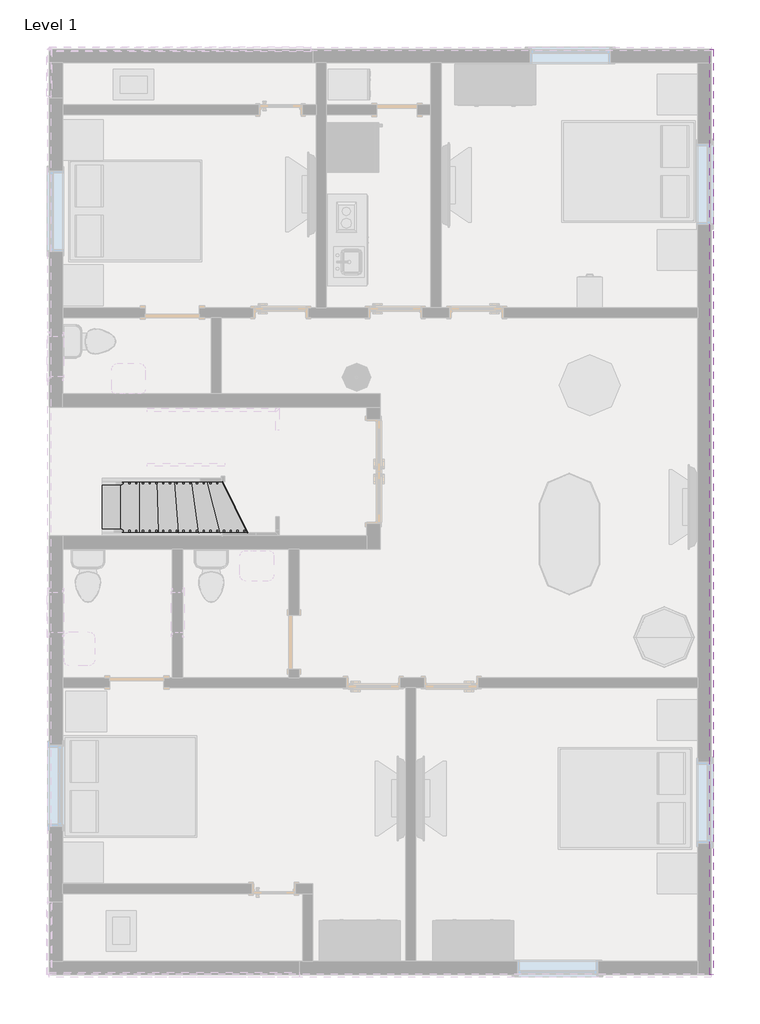
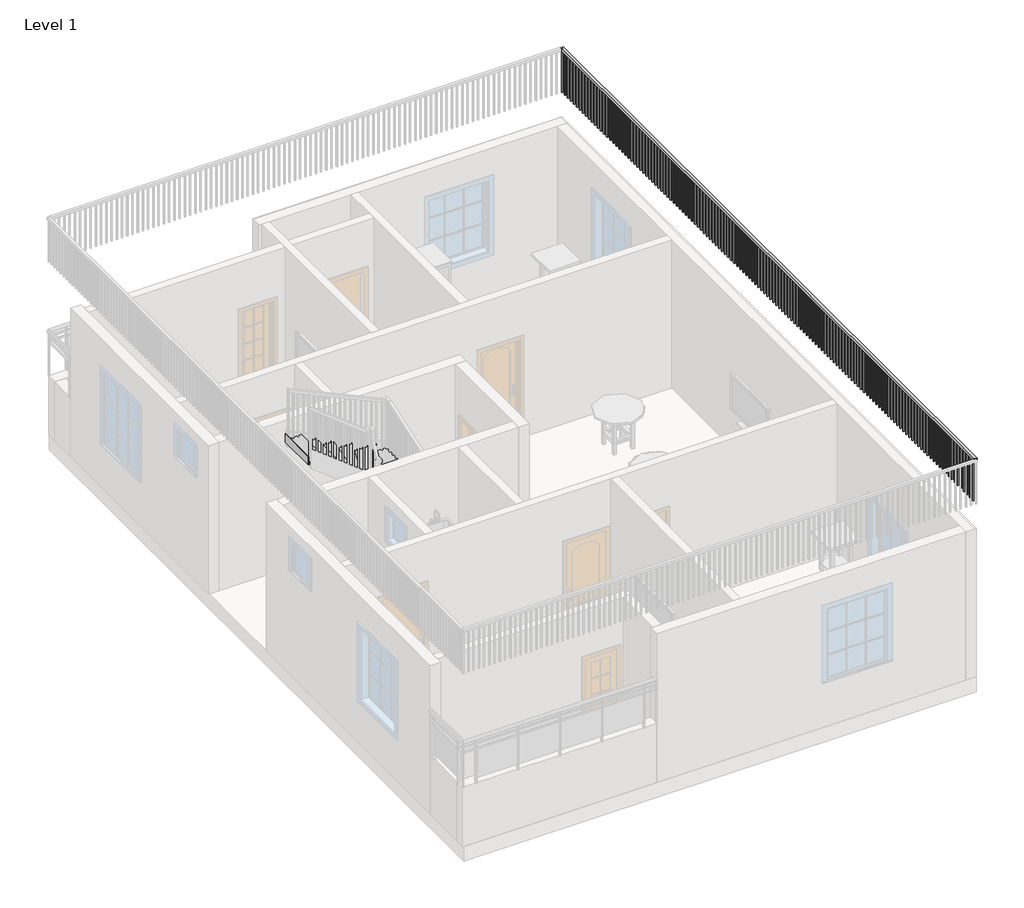
# One storey, part 6 of 7: 1 railing, 1 stair flight.
"""IFC4 building model written with IfcOpenShell, lengths in millimetres."""

from ifc_helpers import new_model, si_unit, frame, origin, place, context, project, spatial, polyline, outline, extrude, transform, mapped, element, save
from components import stair_flight_f4c31f77

model = new_model("IFC4")

# Units and contexts
model_context = context("Model", 3, world=origin())
ifc_project = project(units=[si_unit("LENGTHUNIT", "METRE", prefix="MILLI")], contexts=[model_context])

# Site, building, storey
site = spatial("IfcSite", under=ifc_project)
building = spatial("IfcBuilding", under=site)
storey = spatial("IfcBuildingStorey", under=building, Name="Level 1", Elevation=0.0)

# Railing
placement = place(None, origin())
element("IfcRailing", 1, ObjectType="Handrail - Rectangular", at=placement, inside=storey, context=model_context, shape_type="SweptSolid", body=[
    extrude(outline(polyline([(1501.91525, -1468.5160527), (1451.11525, -1468.5160527), (1451.11525, 12450.6839473), (1501.91525, 12450.6839473), (1501.91525, -1468.5160527)])), frame((0.0, 0.0, 4419.6), z_axis=(0.0, 0.0, 1.0), x_axis=(1.0, 0.0, 0.0)), (0.0, 0.0, 1.0), 50.8),
    extrude(outline(polyline([(1486.04025, 12339.5589473), (1466.99025, 12339.5589473), (1466.99025, 12358.6089473), (1486.04025, 12358.6089473), (1486.04025, 12339.5589473)])), frame((0.0, 0.0, 3556.0), z_axis=(0.0, 0.0, 1.0), x_axis=(1.0, 0.0, 0.0)), (0.0, 0.0, 1.0), 863.6),
    extrude(outline(polyline([(1486.04025, 12237.9589473), (1466.99025, 12237.9589473), (1466.99025, 12257.0089473), (1486.04025, 12257.0089473), (1486.04025, 12237.9589473)])), frame((0.0, 0.0, 3556.0), z_axis=(0.0, 0.0, 1.0), x_axis=(1.0, 0.0, 0.0)), (0.0, 0.0, 1.0), 863.6),
    extrude(outline(polyline([(1486.04025, 12136.3589473), (1466.99025, 12136.3589473), (1466.99025, 12155.4089473), (1486.04025, 12155.4089473), (1486.04025, 12136.3589473)])), frame((0.0, 0.0, 3556.0), z_axis=(0.0, 0.0, 1.0), x_axis=(1.0, 0.0, 0.0)), (0.0, 0.0, 1.0), 863.6),
    extrude(outline(polyline([(1486.04025, 12034.7589473), (1466.99025, 12034.7589473), (1466.99025, 12053.8089473), (1486.04025, 12053.8089473), (1486.04025, 12034.7589473)])), frame((0.0, 0.0, 3556.0), z_axis=(0.0, 0.0, 1.0), x_axis=(1.0, 0.0, 0.0)), (0.0, 0.0, 1.0), 863.6),
    extrude(outline(polyline([(1486.04025, 11933.1589473), (1466.99025, 11933.1589473), (1466.99025, 11952.2089473), (1486.04025, 11952.2089473), (1486.04025, 11933.1589473)])), frame((0.0, 0.0, 3556.0), z_axis=(0.0, 0.0, 1.0), x_axis=(1.0, 0.0, 0.0)), (0.0, 0.0, 1.0), 863.6),
    extrude(outline(polyline([(1486.04025, 11831.5589473), (1466.99025, 11831.5589473), (1466.99025, 11850.6089473), (1486.04025, 11850.6089473), (1486.04025, 11831.5589473)])), frame((0.0, 0.0, 3556.0), z_axis=(0.0, 0.0, 1.0), x_axis=(1.0, 0.0, 0.0)), (0.0, 0.0, 1.0), 863.6),
    extrude(outline(polyline([(1486.04025, 11729.9589473), (1466.99025, 11729.9589473), (1466.99025, 11749.0089473), (1486.04025, 11749.0089473), (1486.04025, 11729.9589473)])), frame((0.0, 0.0, 3556.0), z_axis=(0.0, 0.0, 1.0), x_axis=(1.0, 0.0, 0.0)), (0.0, 0.0, 1.0), 863.6),
    extrude(outline(polyline([(1486.04025, 11628.3589473), (1466.99025, 11628.3589473), (1466.99025, 11647.4089473), (1486.04025, 11647.4089473), (1486.04025, 11628.3589473)])), frame((0.0, 0.0, 3556.0), z_axis=(0.0, 0.0, 1.0), x_axis=(1.0, 0.0, 0.0)), (0.0, 0.0, 1.0), 863.6),
    extrude(outline(polyline([(1486.04025, 11526.7589473), (1466.99025, 11526.7589473), (1466.99025, 11545.8089473), (1486.04025, 11545.8089473), (1486.04025, 11526.7589473)])), frame((0.0, 0.0, 3556.0), z_axis=(0.0, 0.0, 1.0), x_axis=(1.0, 0.0, 0.0)), (0.0, 0.0, 1.0), 863.6),
    extrude(outline(polyline([(1486.04025, 11425.1589473), (1466.99025, 11425.1589473), (1466.99025, 11444.2089473), (1486.04025, 11444.2089473), (1486.04025, 11425.1589473)])), frame((0.0, 0.0, 3556.0), z_axis=(0.0, 0.0, 1.0), x_axis=(1.0, 0.0, 0.0)), (0.0, 0.0, 1.0), 863.6),
    extrude(outline(polyline([(1486.04025, 11323.5589473), (1466.99025, 11323.5589473), (1466.99025, 11342.6089473), (1486.04025, 11342.6089473), (1486.04025, 11323.5589473)])), frame((0.0, 0.0, 3556.0), z_axis=(0.0, 0.0, 1.0), x_axis=(1.0, 0.0, 0.0)), (0.0, 0.0, 1.0), 863.6),
    extrude(outline(polyline([(1486.04025, 11221.9589473), (1466.99025, 11221.9589473), (1466.99025, 11241.0089473), (1486.04025, 11241.0089473), (1486.04025, 11221.9589473)])), frame((0.0, 0.0, 3556.0), z_axis=(0.0, 0.0, 1.0), x_axis=(1.0, 0.0, 0.0)), (0.0, 0.0, 1.0), 863.6),
    extrude(outline(polyline([(1486.04025, 11120.3589473), (1466.99025, 11120.3589473), (1466.99025, 11139.4089473), (1486.04025, 11139.4089473), (1486.04025, 11120.3589473)])), frame((0.0, 0.0, 3556.0), z_axis=(0.0, 0.0, 1.0), x_axis=(1.0, 0.0, 0.0)), (0.0, 0.0, 1.0), 863.6),
    extrude(outline(polyline([(1486.04025, 11018.7589473), (1466.99025, 11018.7589473), (1466.99025, 11037.8089473), (1486.04025, 11037.8089473), (1486.04025, 11018.7589473)])), frame((0.0, 0.0, 3556.0), z_axis=(0.0, 0.0, 1.0), x_axis=(1.0, 0.0, 0.0)), (0.0, 0.0, 1.0), 863.6),
    extrude(outline(polyline([(1486.04025, 10917.1589473), (1466.99025, 10917.1589473), (1466.99025, 10936.2089473), (1486.04025, 10936.2089473), (1486.04025, 10917.1589473)])), frame((0.0, 0.0, 3556.0), z_axis=(0.0, 0.0, 1.0), x_axis=(1.0, 0.0, 0.0)), (0.0, 0.0, 1.0), 863.6),
    extrude(outline(polyline([(1486.04025, 10815.5589473), (1466.99025, 10815.5589473), (1466.99025, 10834.6089473), (1486.04025, 10834.6089473), (1486.04025, 10815.5589473)])), frame((0.0, 0.0, 3556.0), z_axis=(0.0, 0.0, 1.0), x_axis=(1.0, 0.0, 0.0)), (0.0, 0.0, 1.0), 863.6),
    extrude(outline(polyline([(1486.04025, 10713.9589473), (1466.99025, 10713.9589473), (1466.99025, 10733.0089473), (1486.04025, 10733.0089473), (1486.04025, 10713.9589473)])), frame((0.0, 0.0, 3556.0), z_axis=(0.0, 0.0, 1.0), x_axis=(1.0, 0.0, 0.0)), (0.0, 0.0, 1.0), 863.6),
    extrude(outline(polyline([(1486.04025, 10612.3589473), (1466.99025, 10612.3589473), (1466.99025, 10631.4089473), (1486.04025, 10631.4089473), (1486.04025, 10612.3589473)])), frame((0.0, 0.0, 3556.0), z_axis=(0.0, 0.0, 1.0), x_axis=(1.0, 0.0, 0.0)), (0.0, 0.0, 1.0), 863.6),
    extrude(outline(polyline([(1486.04025, 10510.7589473), (1466.99025, 10510.7589473), (1466.99025, 10529.8089473), (1486.04025, 10529.8089473), (1486.04025, 10510.7589473)])), frame((0.0, 0.0, 3556.0), z_axis=(0.0, 0.0, 1.0), x_axis=(1.0, 0.0, 0.0)), (0.0, 0.0, 1.0), 863.6),
    extrude(outline(polyline([(1486.04025, 10409.1589473), (1466.99025, 10409.1589473), (1466.99025, 10428.2089473), (1486.04025, 10428.2089473), (1486.04025, 10409.1589473)])), frame((0.0, 0.0, 3556.0), z_axis=(0.0, 0.0, 1.0), x_axis=(1.0, 0.0, 0.0)), (0.0, 0.0, 1.0), 863.6),
    extrude(outline(polyline([(1486.04025, 10307.5589473), (1466.99025, 10307.5589473), (1466.99025, 10326.6089473), (1486.04025, 10326.6089473), (1486.04025, 10307.5589473)])), frame((0.0, 0.0, 3556.0), z_axis=(0.0, 0.0, 1.0), x_axis=(1.0, 0.0, 0.0)), (0.0, 0.0, 1.0), 863.6),
    extrude(outline(polyline([(1486.04025, 10205.9589473), (1466.99025, 10205.9589473), (1466.99025, 10225.0089473), (1486.04025, 10225.0089473), (1486.04025, 10205.9589473)])), frame((0.0, 0.0, 3556.0), z_axis=(0.0, 0.0, 1.0), x_axis=(1.0, 0.0, 0.0)), (0.0, 0.0, 1.0), 863.6),
    extrude(outline(polyline([(1486.04025, 10104.3589473), (1466.99025, 10104.3589473), (1466.99025, 10123.4089473), (1486.04025, 10123.4089473), (1486.04025, 10104.3589473)])), frame((0.0, 0.0, 3556.0), z_axis=(0.0, 0.0, 1.0), x_axis=(1.0, 0.0, 0.0)), (0.0, 0.0, 1.0), 863.6),
    extrude(outline(polyline([(1486.04025, 10002.7589473), (1466.99025, 10002.7589473), (1466.99025, 10021.8089473), (1486.04025, 10021.8089473), (1486.04025, 10002.7589473)])), frame((0.0, 0.0, 3556.0), z_axis=(0.0, 0.0, 1.0), x_axis=(1.0, 0.0, 0.0)), (0.0, 0.0, 1.0), 863.6),
    extrude(outline(polyline([(1486.04025, 9901.1589473), (1466.99025, 9901.1589473), (1466.99025, 9920.2089473), (1486.04025, 9920.2089473), (1486.04025, 9901.1589473)])), frame((0.0, 0.0, 3556.0), z_axis=(0.0, 0.0, 1.0), x_axis=(1.0, 0.0, 0.0)), (0.0, 0.0, 1.0), 863.6),
    extrude(outline(polyline([(1486.04025, 9799.5589473), (1466.99025, 9799.5589473), (1466.99025, 9818.6089473), (1486.04025, 9818.6089473), (1486.04025, 9799.5589473)])), frame((0.0, 0.0, 3556.0), z_axis=(0.0, 0.0, 1.0), x_axis=(1.0, 0.0, 0.0)), (0.0, 0.0, 1.0), 863.6),
    extrude(outline(polyline([(1486.04025, 9697.9589473), (1466.99025, 9697.9589473), (1466.99025, 9717.0089473), (1486.04025, 9717.0089473), (1486.04025, 9697.9589473)])), frame((0.0, 0.0, 3556.0), z_axis=(0.0, 0.0, 1.0), x_axis=(1.0, 0.0, 0.0)), (0.0, 0.0, 1.0), 863.6),
    extrude(outline(polyline([(1486.04025, 9596.3589473), (1466.99025, 9596.3589473), (1466.99025, 9615.4089473), (1486.04025, 9615.4089473), (1486.04025, 9596.3589473)])), frame((0.0, 0.0, 3556.0), z_axis=(0.0, 0.0, 1.0), x_axis=(1.0, 0.0, 0.0)), (0.0, 0.0, 1.0), 863.6),
    extrude(outline(polyline([(1486.04025, 9494.7589473), (1466.99025, 9494.7589473), (1466.99025, 9513.8089473), (1486.04025, 9513.8089473), (1486.04025, 9494.7589473)])), frame((0.0, 0.0, 3556.0), z_axis=(0.0, 0.0, 1.0), x_axis=(1.0, 0.0, 0.0)), (0.0, 0.0, 1.0), 863.6),
    extrude(outline(polyline([(1486.04025, 9393.1589473), (1466.99025, 9393.1589473), (1466.99025, 9412.2089473), (1486.04025, 9412.2089473), (1486.04025, 9393.1589473)])), frame((0.0, 0.0, 3556.0), z_axis=(0.0, 0.0, 1.0), x_axis=(1.0, 0.0, 0.0)), (0.0, 0.0, 1.0), 863.6),
    extrude(outline(polyline([(1486.04025, 9291.5589473), (1466.99025, 9291.5589473), (1466.99025, 9310.6089473), (1486.04025, 9310.6089473), (1486.04025, 9291.5589473)])), frame((0.0, 0.0, 3556.0), z_axis=(0.0, 0.0, 1.0), x_axis=(1.0, 0.0, 0.0)), (0.0, 0.0, 1.0), 863.6),
    extrude(outline(polyline([(1486.04025, 9189.9589473), (1466.99025, 9189.9589473), (1466.99025, 9209.0089473), (1486.04025, 9209.0089473), (1486.04025, 9189.9589473)])), frame((0.0, 0.0, 3556.0), z_axis=(0.0, 0.0, 1.0), x_axis=(1.0, 0.0, 0.0)), (0.0, 0.0, 1.0), 863.6),
    extrude(outline(polyline([(1486.04025, 9088.3589473), (1466.99025, 9088.3589473), (1466.99025, 9107.4089473), (1486.04025, 9107.4089473), (1486.04025, 9088.3589473)])), frame((0.0, 0.0, 3556.0), z_axis=(0.0, 0.0, 1.0), x_axis=(1.0, 0.0, 0.0)), (0.0, 0.0, 1.0), 863.6),
    extrude(outline(polyline([(1486.04025, 8986.7589473), (1466.99025, 8986.7589473), (1466.99025, 9005.8089473), (1486.04025, 9005.8089473), (1486.04025, 8986.7589473)])), frame((0.0, 0.0, 3556.0), z_axis=(0.0, 0.0, 1.0), x_axis=(1.0, 0.0, 0.0)), (0.0, 0.0, 1.0), 863.6),
    extrude(outline(polyline([(1486.04025, 8885.1589473), (1466.99025, 8885.1589473), (1466.99025, 8904.2089473), (1486.04025, 8904.2089473), (1486.04025, 8885.1589473)])), frame((0.0, 0.0, 3556.0), z_axis=(0.0, 0.0, 1.0), x_axis=(1.0, 0.0, 0.0)), (0.0, 0.0, 1.0), 863.6),
    extrude(outline(polyline([(1486.04025, 8783.5589473), (1466.99025, 8783.5589473), (1466.99025, 8802.6089473), (1486.04025, 8802.6089473), (1486.04025, 8783.5589473)])), frame((0.0, 0.0, 3556.0), z_axis=(0.0, 0.0, 1.0), x_axis=(1.0, 0.0, 0.0)), (0.0, 0.0, 1.0), 863.6),
    extrude(outline(polyline([(1486.04025, 8681.9589473), (1466.99025, 8681.9589473), (1466.99025, 8701.0089473), (1486.04025, 8701.0089473), (1486.04025, 8681.9589473)])), frame((0.0, 0.0, 3556.0), z_axis=(0.0, 0.0, 1.0), x_axis=(1.0, 0.0, 0.0)), (0.0, 0.0, 1.0), 863.6),
    extrude(outline(polyline([(1486.04025, 8580.3589473), (1466.99025, 8580.3589473), (1466.99025, 8599.4089473), (1486.04025, 8599.4089473), (1486.04025, 8580.3589473)])), frame((0.0, 0.0, 3556.0), z_axis=(0.0, 0.0, 1.0), x_axis=(1.0, 0.0, 0.0)), (0.0, 0.0, 1.0), 863.6),
    extrude(outline(polyline([(1486.04025, 8478.7589473), (1466.99025, 8478.7589473), (1466.99025, 8497.8089473), (1486.04025, 8497.8089473), (1486.04025, 8478.7589473)])), frame((0.0, 0.0, 3556.0), z_axis=(0.0, 0.0, 1.0), x_axis=(1.0, 0.0, 0.0)), (0.0, 0.0, 1.0), 863.6),
    extrude(outline(polyline([(1486.04025, 8377.1589473), (1466.99025, 8377.1589473), (1466.99025, 8396.2089473), (1486.04025, 8396.2089473), (1486.04025, 8377.1589473)])), frame((0.0, 0.0, 3556.0), z_axis=(0.0, 0.0, 1.0), x_axis=(1.0, 0.0, 0.0)), (0.0, 0.0, 1.0), 863.6),
    extrude(outline(polyline([(1486.04025, 8275.5589473), (1466.99025, 8275.5589473), (1466.99025, 8294.6089473), (1486.04025, 8294.6089473), (1486.04025, 8275.5589473)])), frame((0.0, 0.0, 3556.0), z_axis=(0.0, 0.0, 1.0), x_axis=(1.0, 0.0, 0.0)), (0.0, 0.0, 1.0), 863.6),
    extrude(outline(polyline([(1486.04025, 8173.9589473), (1466.99025, 8173.9589473), (1466.99025, 8193.0089473), (1486.04025, 8193.0089473), (1486.04025, 8173.9589473)])), frame((0.0, 0.0, 3556.0), z_axis=(0.0, 0.0, 1.0), x_axis=(1.0, 0.0, 0.0)), (0.0, 0.0, 1.0), 863.6),
    extrude(outline(polyline([(1486.04025, 8072.3589473), (1466.99025, 8072.3589473), (1466.99025, 8091.4089473), (1486.04025, 8091.4089473), (1486.04025, 8072.3589473)])), frame((0.0, 0.0, 3556.0), z_axis=(0.0, 0.0, 1.0), x_axis=(1.0, 0.0, 0.0)), (0.0, 0.0, 1.0), 863.6),
    extrude(outline(polyline([(1486.04025, 7970.7589473), (1466.99025, 7970.7589473), (1466.99025, 7989.8089473), (1486.04025, 7989.8089473), (1486.04025, 7970.7589473)])), frame((0.0, 0.0, 3556.0), z_axis=(0.0, 0.0, 1.0), x_axis=(1.0, 0.0, 0.0)), (0.0, 0.0, 1.0), 863.6),
    extrude(outline(polyline([(1486.04025, 7869.1589473), (1466.99025, 7869.1589473), (1466.99025, 7888.2089473), (1486.04025, 7888.2089473), (1486.04025, 7869.1589473)])), frame((0.0, 0.0, 3556.0), z_axis=(0.0, 0.0, 1.0), x_axis=(1.0, 0.0, 0.0)), (0.0, 0.0, 1.0), 863.6),
    extrude(outline(polyline([(1486.04025, 7767.5589473), (1466.99025, 7767.5589473), (1466.99025, 7786.6089473), (1486.04025, 7786.6089473), (1486.04025, 7767.5589473)])), frame((0.0, 0.0, 3556.0), z_axis=(0.0, 0.0, 1.0), x_axis=(1.0, 0.0, 0.0)), (0.0, 0.0, 1.0), 863.6),
    extrude(outline(polyline([(1486.04025, 7665.9589473), (1466.99025, 7665.9589473), (1466.99025, 7685.0089473), (1486.04025, 7685.0089473), (1486.04025, 7665.9589473)])), frame((0.0, 0.0, 3556.0), z_axis=(0.0, 0.0, 1.0), x_axis=(1.0, 0.0, 0.0)), (0.0, 0.0, 1.0), 863.6),
    extrude(outline(polyline([(1486.04025, 7564.3589473), (1466.99025, 7564.3589473), (1466.99025, 7583.4089473), (1486.04025, 7583.4089473), (1486.04025, 7564.3589473)])), frame((0.0, 0.0, 3556.0), z_axis=(0.0, 0.0, 1.0), x_axis=(1.0, 0.0, 0.0)), (0.0, 0.0, 1.0), 863.6),
    extrude(outline(polyline([(1486.04025, 7462.7589473), (1466.99025, 7462.7589473), (1466.99025, 7481.8089473), (1486.04025, 7481.8089473), (1486.04025, 7462.7589473)])), frame((0.0, 0.0, 3556.0), z_axis=(0.0, 0.0, 1.0), x_axis=(1.0, 0.0, 0.0)), (0.0, 0.0, 1.0), 863.6),
    extrude(outline(polyline([(1486.04025, 7361.1589473), (1466.99025, 7361.1589473), (1466.99025, 7380.2089473), (1486.04025, 7380.2089473), (1486.04025, 7361.1589473)])), frame((0.0, 0.0, 3556.0), z_axis=(0.0, 0.0, 1.0), x_axis=(1.0, 0.0, 0.0)), (0.0, 0.0, 1.0), 863.6),
    extrude(outline(polyline([(1486.04025, 7259.5589473), (1466.99025, 7259.5589473), (1466.99025, 7278.6089473), (1486.04025, 7278.6089473), (1486.04025, 7259.5589473)])), frame((0.0, 0.0, 3556.0), z_axis=(0.0, 0.0, 1.0), x_axis=(1.0, 0.0, 0.0)), (0.0, 0.0, 1.0), 863.6),
    extrude(outline(polyline([(1486.04025, 7157.9589473), (1466.99025, 7157.9589473), (1466.99025, 7177.0089473), (1486.04025, 7177.0089473), (1486.04025, 7157.9589473)])), frame((0.0, 0.0, 3556.0), z_axis=(0.0, 0.0, 1.0), x_axis=(1.0, 0.0, 0.0)), (0.0, 0.0, 1.0), 863.6),
    extrude(outline(polyline([(1486.04025, 7056.3589473), (1466.99025, 7056.3589473), (1466.99025, 7075.4089473), (1486.04025, 7075.4089473), (1486.04025, 7056.3589473)])), frame((0.0, 0.0, 3556.0), z_axis=(0.0, 0.0, 1.0), x_axis=(1.0, 0.0, 0.0)), (0.0, 0.0, 1.0), 863.6),
    extrude(outline(polyline([(1486.04025, 6954.7589473), (1466.99025, 6954.7589473), (1466.99025, 6973.8089473), (1486.04025, 6973.8089473), (1486.04025, 6954.7589473)])), frame((0.0, 0.0, 3556.0), z_axis=(0.0, 0.0, 1.0), x_axis=(1.0, 0.0, 0.0)), (0.0, 0.0, 1.0), 863.6),
    extrude(outline(polyline([(1486.04025, 6853.1589473), (1466.99025, 6853.1589473), (1466.99025, 6872.2089473), (1486.04025, 6872.2089473), (1486.04025, 6853.1589473)])), frame((0.0, 0.0, 3556.0), z_axis=(0.0, 0.0, 1.0), x_axis=(1.0, 0.0, 0.0)), (0.0, 0.0, 1.0), 863.6),
    extrude(outline(polyline([(1486.04025, 6751.5589473), (1466.99025, 6751.5589473), (1466.99025, 6770.6089473), (1486.04025, 6770.6089473), (1486.04025, 6751.5589473)])), frame((0.0, 0.0, 3556.0), z_axis=(0.0, 0.0, 1.0), x_axis=(1.0, 0.0, 0.0)), (0.0, 0.0, 1.0), 863.6),
    extrude(outline(polyline([(1486.04025, 6649.9589473), (1466.99025, 6649.9589473), (1466.99025, 6669.0089473), (1486.04025, 6669.0089473), (1486.04025, 6649.9589473)])), frame((0.0, 0.0, 3556.0), z_axis=(0.0, 0.0, 1.0), x_axis=(1.0, 0.0, 0.0)), (0.0, 0.0, 1.0), 863.6),
    extrude(outline(polyline([(1486.04025, 6548.3589473), (1466.99025, 6548.3589473), (1466.99025, 6567.4089473), (1486.04025, 6567.4089473), (1486.04025, 6548.3589473)])), frame((0.0, 0.0, 3556.0), z_axis=(0.0, 0.0, 1.0), x_axis=(1.0, 0.0, 0.0)), (0.0, 0.0, 1.0), 863.6),
    extrude(outline(polyline([(1486.04025, 6446.7589473), (1466.99025, 6446.7589473), (1466.99025, 6465.8089473), (1486.04025, 6465.8089473), (1486.04025, 6446.7589473)])), frame((0.0, 0.0, 3556.0), z_axis=(0.0, 0.0, 1.0), x_axis=(1.0, 0.0, 0.0)), (0.0, 0.0, 1.0), 863.6),
    extrude(outline(polyline([(1486.04025, 6345.1589473), (1466.99025, 6345.1589473), (1466.99025, 6364.2089473), (1486.04025, 6364.2089473), (1486.04025, 6345.1589473)])), frame((0.0, 0.0, 3556.0), z_axis=(0.0, 0.0, 1.0), x_axis=(1.0, 0.0, 0.0)), (0.0, 0.0, 1.0), 863.6),
    extrude(outline(polyline([(1486.04025, 6243.5589473), (1466.99025, 6243.5589473), (1466.99025, 6262.6089473), (1486.04025, 6262.6089473), (1486.04025, 6243.5589473)])), frame((0.0, 0.0, 3556.0), z_axis=(0.0, 0.0, 1.0), x_axis=(1.0, 0.0, 0.0)), (0.0, 0.0, 1.0), 863.6),
    extrude(outline(polyline([(1486.04025, 6141.9589473), (1466.99025, 6141.9589473), (1466.99025, 6161.0089473), (1486.04025, 6161.0089473), (1486.04025, 6141.9589473)])), frame((0.0, 0.0, 3556.0), z_axis=(0.0, 0.0, 1.0), x_axis=(1.0, 0.0, 0.0)), (0.0, 0.0, 1.0), 863.6),
    extrude(outline(polyline([(1486.04025, 6040.3589473), (1466.99025, 6040.3589473), (1466.99025, 6059.4089473), (1486.04025, 6059.4089473), (1486.04025, 6040.3589473)])), frame((0.0, 0.0, 3556.0), z_axis=(0.0, 0.0, 1.0), x_axis=(1.0, 0.0, 0.0)), (0.0, 0.0, 1.0), 863.6),
    extrude(outline(polyline([(1486.04025, 5938.7589473), (1466.99025, 5938.7589473), (1466.99025, 5957.8089473), (1486.04025, 5957.8089473), (1486.04025, 5938.7589473)])), frame((0.0, 0.0, 3556.0), z_axis=(0.0, 0.0, 1.0), x_axis=(1.0, 0.0, 0.0)), (0.0, 0.0, 1.0), 863.6),
    extrude(outline(polyline([(1486.04025, 5837.1589473), (1466.99025, 5837.1589473), (1466.99025, 5856.2089473), (1486.04025, 5856.2089473), (1486.04025, 5837.1589473)])), frame((0.0, 0.0, 3556.0), z_axis=(0.0, 0.0, 1.0), x_axis=(1.0, 0.0, 0.0)), (0.0, 0.0, 1.0), 863.6),
    extrude(outline(polyline([(1486.04025, 5735.5589473), (1466.99025, 5735.5589473), (1466.99025, 5754.6089473), (1486.04025, 5754.6089473), (1486.04025, 5735.5589473)])), frame((0.0, 0.0, 3556.0), z_axis=(0.0, 0.0, 1.0), x_axis=(1.0, 0.0, 0.0)), (0.0, 0.0, 1.0), 863.6),
    extrude(outline(polyline([(1486.04025, 5633.9589473), (1466.99025, 5633.9589473), (1466.99025, 5653.0089473), (1486.04025, 5653.0089473), (1486.04025, 5633.9589473)])), frame((0.0, 0.0, 3556.0), z_axis=(0.0, 0.0, 1.0), x_axis=(1.0, 0.0, 0.0)), (0.0, 0.0, 1.0), 863.6),
    extrude(outline(polyline([(1486.04025, 5532.3589473), (1466.99025, 5532.3589473), (1466.99025, 5551.4089473), (1486.04025, 5551.4089473), (1486.04025, 5532.3589473)])), frame((0.0, 0.0, 3556.0), z_axis=(0.0, 0.0, 1.0), x_axis=(1.0, 0.0, 0.0)), (0.0, 0.0, 1.0), 863.6),
    extrude(outline(polyline([(1486.04025, 5430.7589473), (1466.99025, 5430.7589473), (1466.99025, 5449.8089473), (1486.04025, 5449.8089473), (1486.04025, 5430.7589473)])), frame((0.0, 0.0, 3556.0), z_axis=(0.0, 0.0, 1.0), x_axis=(1.0, 0.0, 0.0)), (0.0, 0.0, 1.0), 863.6),
    extrude(outline(polyline([(1486.04025, 5329.1589473), (1466.99025, 5329.1589473), (1466.99025, 5348.2089473), (1486.04025, 5348.2089473), (1486.04025, 5329.1589473)])), frame((0.0, 0.0, 3556.0), z_axis=(0.0, 0.0, 1.0), x_axis=(1.0, 0.0, 0.0)), (0.0, 0.0, 1.0), 863.6),
    extrude(outline(polyline([(1486.04025, 5227.5589473), (1466.99025, 5227.5589473), (1466.99025, 5246.6089473), (1486.04025, 5246.6089473), (1486.04025, 5227.5589473)])), frame((0.0, 0.0, 3556.0), z_axis=(0.0, 0.0, 1.0), x_axis=(1.0, 0.0, 0.0)), (0.0, 0.0, 1.0), 863.6),
    extrude(outline(polyline([(1486.04025, 5125.9589473), (1466.99025, 5125.9589473), (1466.99025, 5145.0089473), (1486.04025, 5145.0089473), (1486.04025, 5125.9589473)])), frame((0.0, 0.0, 3556.0), z_axis=(0.0, 0.0, 1.0), x_axis=(1.0, 0.0, 0.0)), (0.0, 0.0, 1.0), 863.6),
    extrude(outline(polyline([(1486.04025, 5024.3589473), (1466.99025, 5024.3589473), (1466.99025, 5043.4089473), (1486.04025, 5043.4089473), (1486.04025, 5024.3589473)])), frame((0.0, 0.0, 3556.0), z_axis=(0.0, 0.0, 1.0), x_axis=(1.0, 0.0, 0.0)), (0.0, 0.0, 1.0), 863.6),
    extrude(outline(polyline([(1486.04025, 4922.7589473), (1466.99025, 4922.7589473), (1466.99025, 4941.8089473), (1486.04025, 4941.8089473), (1486.04025, 4922.7589473)])), frame((0.0, 0.0, 3556.0), z_axis=(0.0, 0.0, 1.0), x_axis=(1.0, 0.0, 0.0)), (0.0, 0.0, 1.0), 863.6),
    extrude(outline(polyline([(1486.04025, 4821.1589473), (1466.99025, 4821.1589473), (1466.99025, 4840.2089473), (1486.04025, 4840.2089473), (1486.04025, 4821.1589473)])), frame((0.0, 0.0, 3556.0), z_axis=(0.0, 0.0, 1.0), x_axis=(1.0, 0.0, 0.0)), (0.0, 0.0, 1.0), 863.6),
    extrude(outline(polyline([(1486.04025, 4719.5589473), (1466.99025, 4719.5589473), (1466.99025, 4738.6089473), (1486.04025, 4738.6089473), (1486.04025, 4719.5589473)])), frame((0.0, 0.0, 3556.0), z_axis=(0.0, 0.0, 1.0), x_axis=(1.0, 0.0, 0.0)), (0.0, 0.0, 1.0), 863.6),
    extrude(outline(polyline([(1486.04025, 4617.9589473), (1466.99025, 4617.9589473), (1466.99025, 4637.0089473), (1486.04025, 4637.0089473), (1486.04025, 4617.9589473)])), frame((0.0, 0.0, 3556.0), z_axis=(0.0, 0.0, 1.0), x_axis=(1.0, 0.0, 0.0)), (0.0, 0.0, 1.0), 863.6),
    extrude(outline(polyline([(1486.04025, 4516.3589473), (1466.99025, 4516.3589473), (1466.99025, 4535.4089473), (1486.04025, 4535.4089473), (1486.04025, 4516.3589473)])), frame((0.0, 0.0, 3556.0), z_axis=(0.0, 0.0, 1.0), x_axis=(1.0, 0.0, 0.0)), (0.0, 0.0, 1.0), 863.6),
    extrude(outline(polyline([(1486.04025, 4414.7589473), (1466.99025, 4414.7589473), (1466.99025, 4433.8089473), (1486.04025, 4433.8089473), (1486.04025, 4414.7589473)])), frame((0.0, 0.0, 3556.0), z_axis=(0.0, 0.0, 1.0), x_axis=(1.0, 0.0, 0.0)), (0.0, 0.0, 1.0), 863.6),
    extrude(outline(polyline([(1486.04025, 4313.1589473), (1466.99025, 4313.1589473), (1466.99025, 4332.2089473), (1486.04025, 4332.2089473), (1486.04025, 4313.1589473)])), frame((0.0, 0.0, 3556.0), z_axis=(0.0, 0.0, 1.0), x_axis=(1.0, 0.0, 0.0)), (0.0, 0.0, 1.0), 863.6),
    extrude(outline(polyline([(1486.04025, 4211.5589473), (1466.99025, 4211.5589473), (1466.99025, 4230.6089473), (1486.04025, 4230.6089473), (1486.04025, 4211.5589473)])), frame((0.0, 0.0, 3556.0), z_axis=(0.0, 0.0, 1.0), x_axis=(1.0, 0.0, 0.0)), (0.0, 0.0, 1.0), 863.6),
    extrude(outline(polyline([(1486.04025, 4109.9589473), (1466.99025, 4109.9589473), (1466.99025, 4129.0089473), (1486.04025, 4129.0089473), (1486.04025, 4109.9589473)])), frame((0.0, 0.0, 3556.0), z_axis=(0.0, 0.0, 1.0), x_axis=(1.0, 0.0, 0.0)), (0.0, 0.0, 1.0), 863.6),
    extrude(outline(polyline([(1486.04025, 4008.3589473), (1466.99025, 4008.3589473), (1466.99025, 4027.4089473), (1486.04025, 4027.4089473), (1486.04025, 4008.3589473)])), frame((0.0, 0.0, 3556.0), z_axis=(0.0, 0.0, 1.0), x_axis=(1.0, 0.0, 0.0)), (0.0, 0.0, 1.0), 863.6),
    extrude(outline(polyline([(1486.04025, 3906.7589473), (1466.99025, 3906.7589473), (1466.99025, 3925.8089473), (1486.04025, 3925.8089473), (1486.04025, 3906.7589473)])), frame((0.0, 0.0, 3556.0), z_axis=(0.0, 0.0, 1.0), x_axis=(1.0, 0.0, 0.0)), (0.0, 0.0, 1.0), 863.6),
    extrude(outline(polyline([(1486.04025, 3805.1589473), (1466.99025, 3805.1589473), (1466.99025, 3824.2089473), (1486.04025, 3824.2089473), (1486.04025, 3805.1589473)])), frame((0.0, 0.0, 3556.0), z_axis=(0.0, 0.0, 1.0), x_axis=(1.0, 0.0, 0.0)), (0.0, 0.0, 1.0), 863.6),
    extrude(outline(polyline([(1486.04025, 3703.5589473), (1466.99025, 3703.5589473), (1466.99025, 3722.6089473), (1486.04025, 3722.6089473), (1486.04025, 3703.5589473)])), frame((0.0, 0.0, 3556.0), z_axis=(0.0, 0.0, 1.0), x_axis=(1.0, 0.0, 0.0)), (0.0, 0.0, 1.0), 863.6),
    extrude(outline(polyline([(1486.04025, 3601.9589473), (1466.99025, 3601.9589473), (1466.99025, 3621.0089473), (1486.04025, 3621.0089473), (1486.04025, 3601.9589473)])), frame((0.0, 0.0, 3556.0), z_axis=(0.0, 0.0, 1.0), x_axis=(1.0, 0.0, 0.0)), (0.0, 0.0, 1.0), 863.6),
    extrude(outline(polyline([(1486.04025, 3500.3589473), (1466.99025, 3500.3589473), (1466.99025, 3519.4089473), (1486.04025, 3519.4089473), (1486.04025, 3500.3589473)])), frame((0.0, 0.0, 3556.0), z_axis=(0.0, 0.0, 1.0), x_axis=(1.0, 0.0, 0.0)), (0.0, 0.0, 1.0), 863.6),
    extrude(outline(polyline([(1486.04025, 3398.7589473), (1466.99025, 3398.7589473), (1466.99025, 3417.8089473), (1486.04025, 3417.8089473), (1486.04025, 3398.7589473)])), frame((0.0, 0.0, 3556.0), z_axis=(0.0, 0.0, 1.0), x_axis=(1.0, 0.0, 0.0)), (0.0, 0.0, 1.0), 863.6),
    extrude(outline(polyline([(1486.04025, 3297.1589473), (1466.99025, 3297.1589473), (1466.99025, 3316.2089473), (1486.04025, 3316.2089473), (1486.04025, 3297.1589473)])), frame((0.0, 0.0, 3556.0), z_axis=(0.0, 0.0, 1.0), x_axis=(1.0, 0.0, 0.0)), (0.0, 0.0, 1.0), 863.6),
    extrude(outline(polyline([(1486.04025, 3195.5589473), (1466.99025, 3195.5589473), (1466.99025, 3214.6089473), (1486.04025, 3214.6089473), (1486.04025, 3195.5589473)])), frame((0.0, 0.0, 3556.0), z_axis=(0.0, 0.0, 1.0), x_axis=(1.0, 0.0, 0.0)), (0.0, 0.0, 1.0), 863.6),
    extrude(outline(polyline([(1486.04025, 3093.9589473), (1466.99025, 3093.9589473), (1466.99025, 3113.0089473), (1486.04025, 3113.0089473), (1486.04025, 3093.9589473)])), frame((0.0, 0.0, 3556.0), z_axis=(0.0, 0.0, 1.0), x_axis=(1.0, 0.0, 0.0)), (0.0, 0.0, 1.0), 863.6),
    extrude(outline(polyline([(1486.04025, 2992.3589473), (1466.99025, 2992.3589473), (1466.99025, 3011.4089473), (1486.04025, 3011.4089473), (1486.04025, 2992.3589473)])), frame((0.0, 0.0, 3556.0), z_axis=(0.0, 0.0, 1.0), x_axis=(1.0, 0.0, 0.0)), (0.0, 0.0, 1.0), 863.6),
    extrude(outline(polyline([(1486.04025, 2890.7589473), (1466.99025, 2890.7589473), (1466.99025, 2909.8089473), (1486.04025, 2909.8089473), (1486.04025, 2890.7589473)])), frame((0.0, 0.0, 3556.0), z_axis=(0.0, 0.0, 1.0), x_axis=(1.0, 0.0, 0.0)), (0.0, 0.0, 1.0), 863.6),
    extrude(outline(polyline([(1486.04025, 2789.1589473), (1466.99025, 2789.1589473), (1466.99025, 2808.2089473), (1486.04025, 2808.2089473), (1486.04025, 2789.1589473)])), frame((0.0, 0.0, 3556.0), z_axis=(0.0, 0.0, 1.0), x_axis=(1.0, 0.0, 0.0)), (0.0, 0.0, 1.0), 863.6),
    extrude(outline(polyline([(1486.04025, 2687.5589473), (1466.99025, 2687.5589473), (1466.99025, 2706.6089473), (1486.04025, 2706.6089473), (1486.04025, 2687.5589473)])), frame((0.0, 0.0, 3556.0), z_axis=(0.0, 0.0, 1.0), x_axis=(1.0, 0.0, 0.0)), (0.0, 0.0, 1.0), 863.6),
    extrude(outline(polyline([(1486.04025, 2585.9589473), (1466.99025, 2585.9589473), (1466.99025, 2605.0089473), (1486.04025, 2605.0089473), (1486.04025, 2585.9589473)])), frame((0.0, 0.0, 3556.0), z_axis=(0.0, 0.0, 1.0), x_axis=(1.0, 0.0, 0.0)), (0.0, 0.0, 1.0), 863.6),
    extrude(outline(polyline([(1486.04025, 2484.3589473), (1466.99025, 2484.3589473), (1466.99025, 2503.4089473), (1486.04025, 2503.4089473), (1486.04025, 2484.3589473)])), frame((0.0, 0.0, 3556.0), z_axis=(0.0, 0.0, 1.0), x_axis=(1.0, 0.0, 0.0)), (0.0, 0.0, 1.0), 863.6),
    extrude(outline(polyline([(1486.04025, 2382.7589473), (1466.99025, 2382.7589473), (1466.99025, 2401.8089473), (1486.04025, 2401.8089473), (1486.04025, 2382.7589473)])), frame((0.0, 0.0, 3556.0), z_axis=(0.0, 0.0, 1.0), x_axis=(1.0, 0.0, 0.0)), (0.0, 0.0, 1.0), 863.6),
    extrude(outline(polyline([(1486.04025, 2281.1589473), (1466.99025, 2281.1589473), (1466.99025, 2300.2089473), (1486.04025, 2300.2089473), (1486.04025, 2281.1589473)])), frame((0.0, 0.0, 3556.0), z_axis=(0.0, 0.0, 1.0), x_axis=(1.0, 0.0, 0.0)), (0.0, 0.0, 1.0), 863.6),
    extrude(outline(polyline([(1486.04025, 2179.5589473), (1466.99025, 2179.5589473), (1466.99025, 2198.6089473), (1486.04025, 2198.6089473), (1486.04025, 2179.5589473)])), frame((0.0, 0.0, 3556.0), z_axis=(0.0, 0.0, 1.0), x_axis=(1.0, 0.0, 0.0)), (0.0, 0.0, 1.0), 863.6),
    extrude(outline(polyline([(1486.04025, 2077.9589473), (1466.99025, 2077.9589473), (1466.99025, 2097.0089473), (1486.04025, 2097.0089473), (1486.04025, 2077.9589473)])), frame((0.0, 0.0, 3556.0), z_axis=(0.0, 0.0, 1.0), x_axis=(1.0, 0.0, 0.0)), (0.0, 0.0, 1.0), 863.6),
    extrude(outline(polyline([(1486.04025, 1976.3589473), (1466.99025, 1976.3589473), (1466.99025, 1995.4089473), (1486.04025, 1995.4089473), (1486.04025, 1976.3589473)])), frame((0.0, 0.0, 3556.0), z_axis=(0.0, 0.0, 1.0), x_axis=(1.0, 0.0, 0.0)), (0.0, 0.0, 1.0), 863.6),
    extrude(outline(polyline([(1486.04025, 1874.7589473), (1466.99025, 1874.7589473), (1466.99025, 1893.8089473), (1486.04025, 1893.8089473), (1486.04025, 1874.7589473)])), frame((0.0, 0.0, 3556.0), z_axis=(0.0, 0.0, 1.0), x_axis=(1.0, 0.0, 0.0)), (0.0, 0.0, 1.0), 863.6),
    extrude(outline(polyline([(1486.04025, 1773.1589473), (1466.99025, 1773.1589473), (1466.99025, 1792.2089473), (1486.04025, 1792.2089473), (1486.04025, 1773.1589473)])), frame((0.0, 0.0, 3556.0), z_axis=(0.0, 0.0, 1.0), x_axis=(1.0, 0.0, 0.0)), (0.0, 0.0, 1.0), 863.6),
    extrude(outline(polyline([(1486.04025, 1671.5589473), (1466.99025, 1671.5589473), (1466.99025, 1690.6089473), (1486.04025, 1690.6089473), (1486.04025, 1671.5589473)])), frame((0.0, 0.0, 3556.0), z_axis=(0.0, 0.0, 1.0), x_axis=(1.0, 0.0, 0.0)), (0.0, 0.0, 1.0), 863.6),
    extrude(outline(polyline([(1486.04025, 1569.9589473), (1466.99025, 1569.9589473), (1466.99025, 1589.0089473), (1486.04025, 1589.0089473), (1486.04025, 1569.9589473)])), frame((0.0, 0.0, 3556.0), z_axis=(0.0, 0.0, 1.0), x_axis=(1.0, 0.0, 0.0)), (0.0, 0.0, 1.0), 863.6),
    extrude(outline(polyline([(1486.04025, 1468.3589473), (1466.99025, 1468.3589473), (1466.99025, 1487.4089473), (1486.04025, 1487.4089473), (1486.04025, 1468.3589473)])), frame((0.0, 0.0, 3556.0), z_axis=(0.0, 0.0, 1.0), x_axis=(1.0, 0.0, 0.0)), (0.0, 0.0, 1.0), 863.6),
    extrude(outline(polyline([(1486.04025, 1366.7589473), (1466.99025, 1366.7589473), (1466.99025, 1385.8089473), (1486.04025, 1385.8089473), (1486.04025, 1366.7589473)])), frame((0.0, 0.0, 3556.0), z_axis=(0.0, 0.0, 1.0), x_axis=(1.0, 0.0, 0.0)), (0.0, 0.0, 1.0), 863.6),
    extrude(outline(polyline([(1486.04025, 1265.1589473), (1466.99025, 1265.1589473), (1466.99025, 1284.2089473), (1486.04025, 1284.2089473), (1486.04025, 1265.1589473)])), frame((0.0, 0.0, 3556.0), z_axis=(0.0, 0.0, 1.0), x_axis=(1.0, 0.0, 0.0)), (0.0, 0.0, 1.0), 863.6),
    extrude(outline(polyline([(1486.04025, 1163.5589473), (1466.99025, 1163.5589473), (1466.99025, 1182.6089473), (1486.04025, 1182.6089473), (1486.04025, 1163.5589473)])), frame((0.0, 0.0, 3556.0), z_axis=(0.0, 0.0, 1.0), x_axis=(1.0, 0.0, 0.0)), (0.0, 0.0, 1.0), 863.6),
    extrude(outline(polyline([(1486.04025, 1061.9589473), (1466.99025, 1061.9589473), (1466.99025, 1081.0089473), (1486.04025, 1081.0089473), (1486.04025, 1061.9589473)])), frame((0.0, 0.0, 3556.0), z_axis=(0.0, 0.0, 1.0), x_axis=(1.0, 0.0, 0.0)), (0.0, 0.0, 1.0), 863.6),
    extrude(outline(polyline([(1486.04025, 960.3589473), (1466.99025, 960.3589473), (1466.99025, 979.4089473), (1486.04025, 979.4089473), (1486.04025, 960.3589473)])), frame((0.0, 0.0, 3556.0), z_axis=(0.0, 0.0, 1.0), x_axis=(1.0, 0.0, 0.0)), (0.0, 0.0, 1.0), 863.6),
    extrude(outline(polyline([(1486.04025, 858.7589473), (1466.99025, 858.7589473), (1466.99025, 877.8089473), (1486.04025, 877.8089473), (1486.04025, 858.7589473)])), frame((0.0, 0.0, 3556.0), z_axis=(0.0, 0.0, 1.0), x_axis=(1.0, 0.0, 0.0)), (0.0, 0.0, 1.0), 863.6),
    extrude(outline(polyline([(1486.04025, 757.1589473), (1466.99025, 757.1589473), (1466.99025, 776.2089473), (1486.04025, 776.2089473), (1486.04025, 757.1589473)])), frame((0.0, 0.0, 3556.0), z_axis=(0.0, 0.0, 1.0), x_axis=(1.0, 0.0, 0.0)), (0.0, 0.0, 1.0), 863.6),
    extrude(outline(polyline([(1486.04025, 655.5589473), (1466.99025, 655.5589473), (1466.99025, 674.6089473), (1486.04025, 674.6089473), (1486.04025, 655.5589473)])), frame((0.0, 0.0, 3556.0), z_axis=(0.0, 0.0, 1.0), x_axis=(1.0, 0.0, 0.0)), (0.0, 0.0, 1.0), 863.6),
    extrude(outline(polyline([(1486.04025, 553.9589473), (1466.99025, 553.9589473), (1466.99025, 573.0089473), (1486.04025, 573.0089473), (1486.04025, 553.9589473)])), frame((0.0, 0.0, 3556.0), z_axis=(0.0, 0.0, 1.0), x_axis=(1.0, 0.0, 0.0)), (0.0, 0.0, 1.0), 863.6),
    extrude(outline(polyline([(1486.04025, 452.3589473), (1466.99025, 452.3589473), (1466.99025, 471.4089473), (1486.04025, 471.4089473), (1486.04025, 452.3589473)])), frame((0.0, 0.0, 3556.0), z_axis=(0.0, 0.0, 1.0), x_axis=(1.0, 0.0, 0.0)), (0.0, 0.0, 1.0), 863.6),
    extrude(outline(polyline([(1486.04025, 350.7589473), (1466.99025, 350.7589473), (1466.99025, 369.8089473), (1486.04025, 369.8089473), (1486.04025, 350.7589473)])), frame((0.0, 0.0, 3556.0), z_axis=(0.0, 0.0, 1.0), x_axis=(1.0, 0.0, 0.0)), (0.0, 0.0, 1.0), 863.6),
    extrude(outline(polyline([(1486.04025, 249.1589473), (1466.99025, 249.1589473), (1466.99025, 268.2089473), (1486.04025, 268.2089473), (1486.04025, 249.1589473)])), frame((0.0, 0.0, 3556.0), z_axis=(0.0, 0.0, 1.0), x_axis=(1.0, 0.0, 0.0)), (0.0, 0.0, 1.0), 863.6),
    extrude(outline(polyline([(1486.04025, 147.5589473), (1466.99025, 147.5589473), (1466.99025, 166.6089473), (1486.04025, 166.6089473), (1486.04025, 147.5589473)])), frame((0.0, 0.0, 3556.0), z_axis=(0.0, 0.0, 1.0), x_axis=(1.0, 0.0, 0.0)), (0.0, 0.0, 1.0), 863.6),
    extrude(outline(polyline([(1486.04025, 45.9589473), (1466.99025, 45.9589473), (1466.99025, 65.0089473), (1486.04025, 65.0089473), (1486.04025, 45.9589473)])), frame((0.0, 0.0, 3556.0), z_axis=(0.0, 0.0, 1.0), x_axis=(1.0, 0.0, 0.0)), (0.0, 0.0, 1.0), 863.6),
    extrude(outline(polyline([(1486.04025, -55.6410527), (1466.99025, -55.6410527), (1466.99025, -36.5910527), (1486.04025, -36.5910527), (1486.04025, -55.6410527)])), frame((0.0, 0.0, 3556.0), z_axis=(0.0, 0.0, 1.0), x_axis=(1.0, 0.0, 0.0)), (0.0, 0.0, 1.0), 863.6),
    extrude(outline(polyline([(1486.04025, -157.2410527), (1466.99025, -157.2410527), (1466.99025, -138.1910527), (1486.04025, -138.1910527), (1486.04025, -157.2410527)])), frame((0.0, 0.0, 3556.0), z_axis=(0.0, 0.0, 1.0), x_axis=(1.0, 0.0, 0.0)), (0.0, 0.0, 1.0), 863.6),
    extrude(outline(polyline([(1486.04025, -258.8410527), (1466.99025, -258.8410527), (1466.99025, -239.7910527), (1486.04025, -239.7910527), (1486.04025, -258.8410527)])), frame((0.0, 0.0, 3556.0), z_axis=(0.0, 0.0, 1.0), x_axis=(1.0, 0.0, 0.0)), (0.0, 0.0, 1.0), 863.6),
    extrude(outline(polyline([(1486.04025, -360.4410527), (1466.99025, -360.4410527), (1466.99025, -341.3910527), (1486.04025, -341.3910527), (1486.04025, -360.4410527)])), frame((0.0, 0.0, 3556.0), z_axis=(0.0, 0.0, 1.0), x_axis=(1.0, 0.0, 0.0)), (0.0, 0.0, 1.0), 863.6),
    extrude(outline(polyline([(1486.04025, -462.0410527), (1466.99025, -462.0410527), (1466.99025, -442.9910527), (1486.04025, -442.9910527), (1486.04025, -462.0410527)])), frame((0.0, 0.0, 3556.0), z_axis=(0.0, 0.0, 1.0), x_axis=(1.0, 0.0, 0.0)), (0.0, 0.0, 1.0), 863.6),
    extrude(outline(polyline([(1486.04025, -563.6410527), (1466.99025, -563.6410527), (1466.99025, -544.5910527), (1486.04025, -544.5910527), (1486.04025, -563.6410527)])), frame((0.0, 0.0, 3556.0), z_axis=(0.0, 0.0, 1.0), x_axis=(1.0, 0.0, 0.0)), (0.0, 0.0, 1.0), 863.6),
    extrude(outline(polyline([(1486.04025, -665.2410527), (1466.99025, -665.2410527), (1466.99025, -646.1910527), (1486.04025, -646.1910527), (1486.04025, -665.2410527)])), frame((0.0, 0.0, 3556.0), z_axis=(0.0, 0.0, 1.0), x_axis=(1.0, 0.0, 0.0)), (0.0, 0.0, 1.0), 863.6),
    extrude(outline(polyline([(1486.04025, -766.8410527), (1466.99025, -766.8410527), (1466.99025, -747.7910527), (1486.04025, -747.7910527), (1486.04025, -766.8410527)])), frame((0.0, 0.0, 3556.0), z_axis=(0.0, 0.0, 1.0), x_axis=(1.0, 0.0, 0.0)), (0.0, 0.0, 1.0), 863.6),
    extrude(outline(polyline([(1486.04025, -868.4410527), (1466.99025, -868.4410527), (1466.99025, -849.3910527), (1486.04025, -849.3910527), (1486.04025, -868.4410527)])), frame((0.0, 0.0, 3556.0), z_axis=(0.0, 0.0, 1.0), x_axis=(1.0, 0.0, 0.0)), (0.0, 0.0, 1.0), 863.6),
    extrude(outline(polyline([(1486.04025, -970.0410527), (1466.99025, -970.0410527), (1466.99025, -950.9910527), (1486.04025, -950.9910527), (1486.04025, -970.0410527)])), frame((0.0, 0.0, 3556.0), z_axis=(0.0, 0.0, 1.0), x_axis=(1.0, 0.0, 0.0)), (0.0, 0.0, 1.0), 863.6),
    extrude(outline(polyline([(1486.04025, -1071.6410527), (1466.99025, -1071.6410527), (1466.99025, -1052.5910527), (1486.04025, -1052.5910527), (1486.04025, -1071.6410527)])), frame((0.0, 0.0, 3556.0), z_axis=(0.0, 0.0, 1.0), x_axis=(1.0, 0.0, 0.0)), (0.0, 0.0, 1.0), 863.6),
    extrude(outline(polyline([(1486.04025, -1173.2410527), (1466.99025, -1173.2410527), (1466.99025, -1154.1910527), (1486.04025, -1154.1910527), (1486.04025, -1173.2410527)])), frame((0.0, 0.0, 3556.0), z_axis=(0.0, 0.0, 1.0), x_axis=(1.0, 0.0, 0.0)), (0.0, 0.0, 1.0), 863.6),
    extrude(outline(polyline([(1486.04025, -1274.8410527), (1466.99025, -1274.8410527), (1466.99025, -1255.7910527), (1486.04025, -1255.7910527), (1486.04025, -1274.8410527)])), frame((0.0, 0.0, 3556.0), z_axis=(0.0, 0.0, 1.0), x_axis=(1.0, 0.0, 0.0)), (0.0, 0.0, 1.0), 863.6),
    extrude(outline(polyline([(1486.04025, -1376.4410527), (1466.99025, -1376.4410527), (1466.99025, -1357.3910527), (1486.04025, -1357.3910527), (1486.04025, -1376.4410527)])), frame((0.0, 0.0, 3556.0), z_axis=(0.0, 0.0, 1.0), x_axis=(1.0, 0.0, 0.0)), (0.0, 0.0, 1.0), 863.6),
    extrude(outline(polyline([(1486.04025, 12431.6339473), (1466.99025, 12431.6339473), (1466.99025, 12450.6839473), (1486.04025, 12450.6839473), (1486.04025, 12431.6339473)])), frame((0.0, 0.0, 3556.0), z_axis=(0.0, 0.0, 1.0), x_axis=(1.0, 0.0, 0.0)), (0.0, 0.0, 1.0), 863.6),
    extrude(outline(polyline([(1486.04025, -1468.5160527), (1466.99025, -1468.5160527), (1466.99025, -1449.4660527), (1486.04025, -1449.4660527), (1486.04025, -1468.5160527)])), frame((0.0, 0.0, 3556.0), z_axis=(0.0, 0.0, 1.0), x_axis=(1.0, 0.0, 0.0)), (0.0, 0.0, 1.0), 863.6),
])

# Stair flight
stair_flight_shape = stair_flight_f4c31f77(model_context)
element("IfcStairFlight", 2, ObjectType="2\" Tread 1\" Nosing 1/4\" Riser", at=placement, inside=storey, context=model_context, shape_type="MappedRepresentation", body=[
    mapped(stair_flight_shape, transform((0.0, 0.0, 0.0), x_axis=(1.0, 0.0, 0.0), y_axis=(0.0, 1.0, 0.0), z_axis=(0.0, 0.0, 1.0))),
])

save(model, "model.ifc")

# Revit data of these elements
# Type "Handrail - Rectangular"
#   Assembly Code = "C2010400"
#   built-in parameter 1008612 = 0.0416667 (stored number, unit not read)
#   built-in parameter 1008611 = 0.0416667 (stored number, unit not read)
#   built-in parameter 1008609 = 0.333333 (stored number, unit not read)
#   built-in parameter 1008604 = 0.166667 (stored number, unit not read)
#   built-in parameter 1008603 = 0.166667 (stored number, unit not read)
#   Railing Height = 3' - 0"
#   built-in parameter 1008630 = 2
#   built-in parameter 1008610 = 2
#   built-in parameter 1008618 = Baluster - Square : 3/4"
# Element 1 (IfcRailing, "Handrail - Rectangular")
#   built-in parameter 1008621 = 11.6667 (stored number, unit not read)
#   Phase Created = New Construction
# Element 2 (IfcStairFlight, "2\" Tread 1\" Nosing 1/4\" Riser")
#   Phase Created = New Construction
